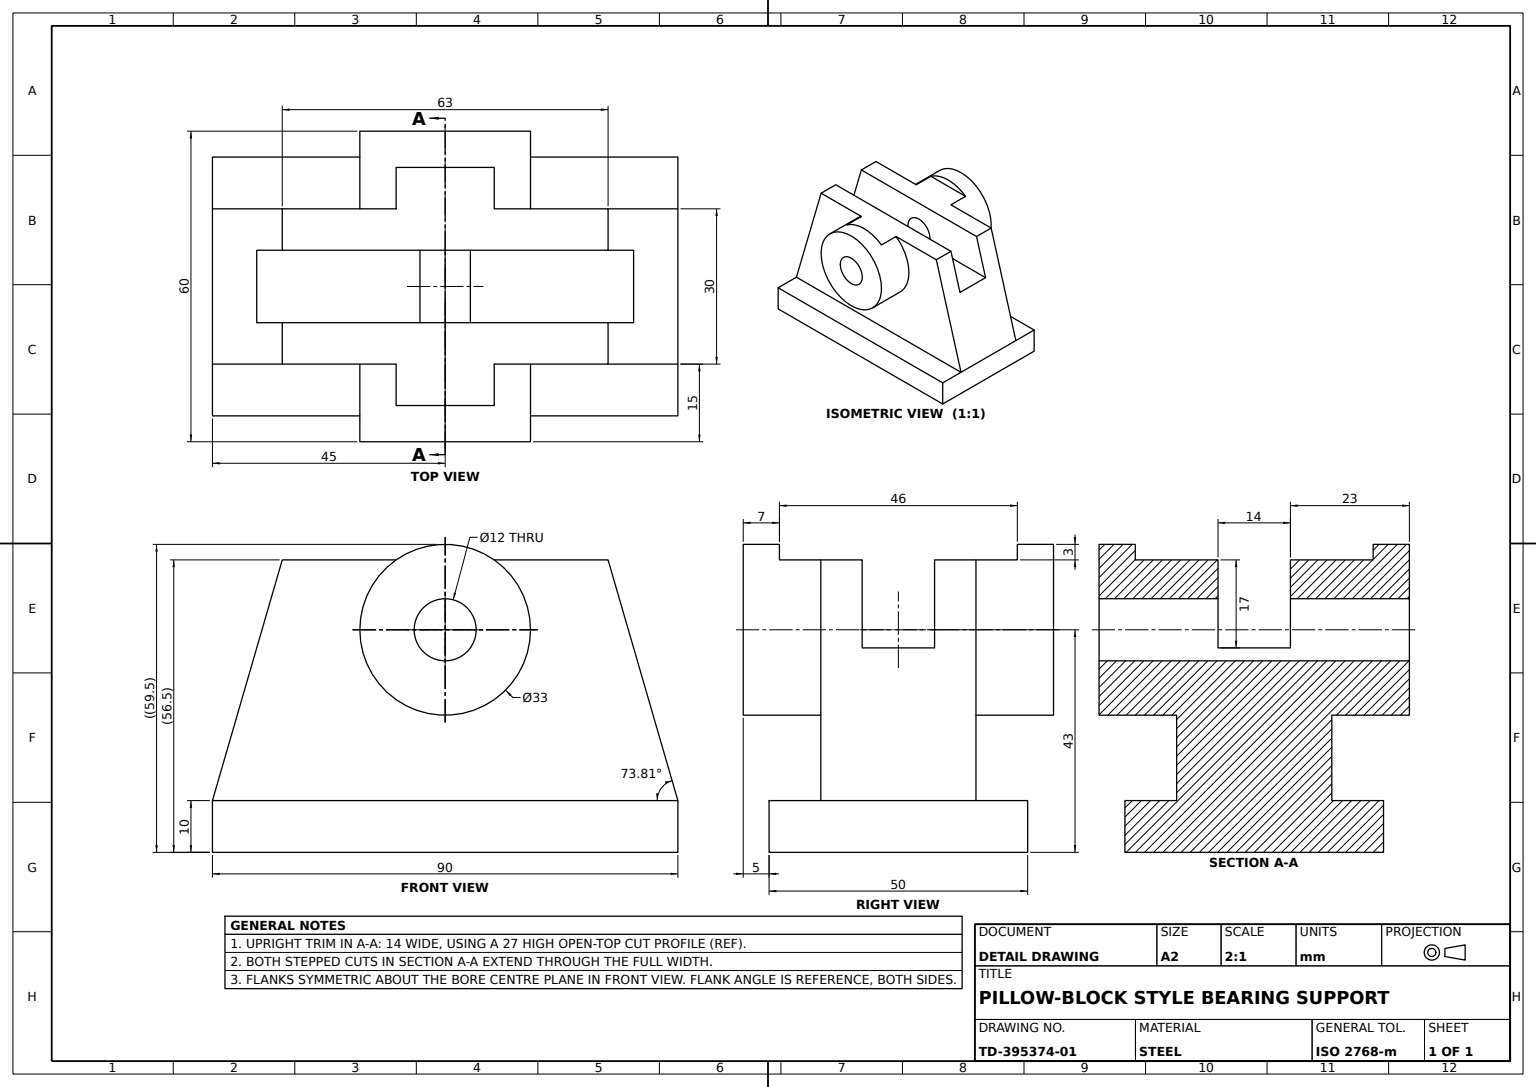
SolidWorks part; units mm, degrees
material "Plain Carbon Steel"
ref_plane "Front Plane" through (0, 0, 0) normal (0, 0, 1) x (1, 0, 0)
ref_plane "Top Plane" through (0, 0, 0) normal (0, 1, 0) x (1, 0, 0)
ref_plane "Right Plane" through (0, 0, 0) normal (1, 0, 0) x (0, 0, -1)
sketch "Base Plate Sketch" plane through (0, 0, 0) normal (0, 1, 0) x (1, 0, 0)
  line L1 (-25, 45) -> (25, 45)
  line L2 (-25, 45) -> (-25, -45)
  line L3 (-25, -45) -> (25, -45)
  line L4 (25, 45) -> (25, -45)
  line L5 (-25, 45) -> (25, -45) construction
  line L6 (-25, -45) -> (25, 45) construction
  point P0 (0, 0)
  dimension "D1" = 50
  dimension "D2" = 90
extrude "Base Plate 90x50x10" add sketch "Base Plate Sketch" along normal blind 10
sketch "Upright Profile Sketch" plane through (0, 10, 0) normal (0, 1, 0) x (1, 0, 0)
  line L0 (-25, -45) -> (25, -45) construction
  line L1 (-15, 45) -> (15, 45)
  line L2 (-15, 45) -> (-15, -45)
  line L3 (-15, -45) -> (15, -45)
  line L4 (15, 45) -> (15, -45)
  line L5 (-15, 45) -> (15, -45) construction
  line L6 (-15, -45) -> (15, 45) construction
  point P0 (0, 0)
  dimension "D1" = 30
extrude "Tapered Upright" add sketch "Upright Profile Sketch" along normal blind 56.5
sketch "Upright Trim Sketch" plane through (0, 0, 45) normal (0, 0, 1) x (1, 0, 0)
  line L0 (-15, 66.5) -> (15, 66.5) construction
  line L1 (7, 39.5) -> (-7, 39.5)
  line L2 (7, 39.5) -> (7, 66.5)
  line L3 (7, 66.5) -> (-7, 66.5)
  line L4 (-7, 39.5) -> (-7, 66.5)
  line L5 (7, 39.5) -> (-7, 66.5) construction
  line L6 (7, 66.5) -> (-7, 39.5) construction
  point P0 (0, 53)
  dimension "D1" = 14
  dimension "D2" = 0
  dimension "D3" = 27
extrude "Upright Trim Cut" cut sketch "Upright Trim Sketch" against normal through all
sketch "Bearing Boss Sketch" plane through (0, 0, 0) normal (1, 0, 0) x (0, 0, -1)
  line L0 (-45, 0) -> (45, 0) construction
  line L1 (45, 66.5) -> (45, 10) construction
  circle A0 centre (0, 43) radius 6
  circle A1 centre (0, 43) radius 16.5
  dimension "D1" = 12
  dimension "D2" = 33
  dimension "D3" = 43
  dimension "D4" = 45
extrude "Bearing Boss" add sketch "Bearing Boss Sketch" along normal mid plane 60
sketch "Centre Slot Sketch" plane through (0, 0, 0) normal (0, 0, 1) x (1, 0, 0)
  line L0 (-15, 59.5) -> (-30, 59.5) construction
  line L1 (-23, 66.5) -> (23, 66.5)
  line L2 (-23, 66.5) -> (-23, 56.5)
  line L3 (-23, 56.5) -> (23, 56.5)
  line L4 (23, 66.5) -> (23, 56.5)
  dimension "D1" = 46
  dimension "D2" = 23
  dimension "D3" = 10
  dimension "D4" = 7
extrude "Centre Slot Cut" cut sketch "Centre Slot Sketch" against normal mid plane 130
sketch "Top Slot Sketch" plane through (0, 0, 0) normal (1, 0, 0) x (0, 0, -1)
  line L1 (-9.4868, 56.5) -> (-45, 56.5) construction
  line L2 (45, 56.5) -> (9.4868, 56.5) construction
  line L3 (-31.5, 56.5) -> (-45, 10)
  line L4 (-45, 10) -> (-45, 56.5)
  line L5 (-45, 56.5) -> (-31.5, 56.5)
  line L6 (31.5, 56.5) -> (45, 10)
  line L7 (45, 10) -> (45, 56.5)
  line L8 (45, 56.5) -> (31.5, 56.5)
  dimension "D1" = 63
  dimension "D2" = 31.5
extrude "Top Slot Cut" cut sketch "Top Slot Sketch" against normal mid plane 130
sketch "Bearing Bore Sketch" plane through (-15, 0, 0) normal (-1, 0, 0) x (0, 0, 1)
  circle A0 centre (0, 43) radius 6 construction
  circle A1 centre (0, 43) radius 6
extrude "Bearing Bore Through" cut sketch "Bearing Bore Sketch" against normal mid plane 130
sketch "Boss Notch Sketch" plane through (0, 0, 0) normal (0, 0, 1) x (1, 0, 0)
  line L4 (7, 39.5) -> (7, 56.5)
  line L5 (7, 56.5) -> (-7, 56.5)
  line L6 (-7, 56.5) -> (-7, 39.5)
  line L7 (-7, 39.5) -> (7, 39.5)
  line L8 (7, 39.5) -> (7, 56.5)
  line L9 (7, 56.5) -> (-7, 56.5)
  line L10 (-7, 56.5) -> (-7, 39.5)
  line L11 (-7, 39.5) -> (7, 39.5)
  dimension "D1" = 0
extrude "Boss Notch Cut" cut sketch "Boss Notch Sketch" against normal mid plane 130
